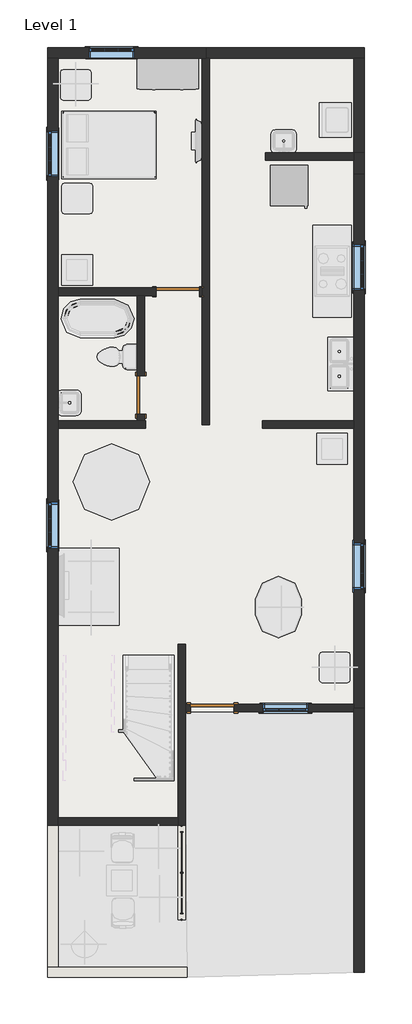
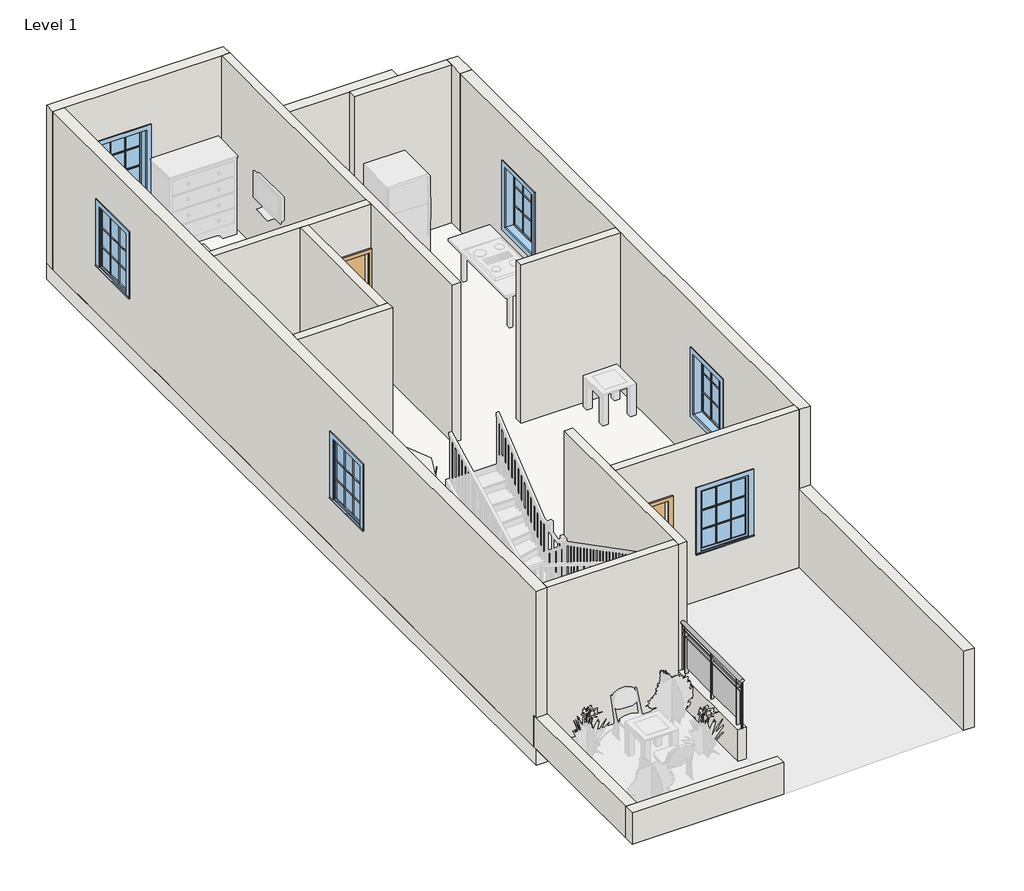
# One storey, part 1 of 3: 19 walls, 6 windows, 3 doors, 1 railing, 1 slab.
"""IFC4 building model written with IfcOpenShell, lengths in millimetres."""

from ifc_helpers import new_model, si_unit, point, frame, origin, origin_with_axes, place, context, project, spatial, polyline, ellipse_curve, trimmed, outline, extrude, faceted_brep, transform, mapped, element, save
from ifc_brep_helpers import plane_surface, extruded_surface, advanced_brep
from components import door_255cab33, door_b6e9fca3, door_99d96fc5, window_29c06734, window_5c190c7e

model = new_model("IFC4")

# Units and contexts
model_context = context("Model", 3, world=origin())
ifc_project = project(units=[si_unit("LENGTHUNIT", "METRE", prefix="MILLI")], contexts=[model_context])

# Site, building, storey
site = spatial("IfcSite", under=ifc_project)
building = spatial("IfcBuilding", under=site)
storey = spatial("IfcBuildingStorey", under=building, Name="Level 1", Elevation=0.0)

# Doors
placement = place(None, origin())
door_shape = door_255cab33(model_context)
element("IfcDoor", 1, ObjectType="Single-Flush : 30\" x 80\"", at=placement, inside=storey, context=model_context, shape_type="MappedRepresentation", body=[
    mapped(door_shape, transform((-1163.5479637, 6058.6104001, 0.0), x_axis=(0.0, -1.0, 0.0), y_axis=(1.0, 0.0, 0.0), z_axis=(0.0, 0.0, 1.0))),
])
door_2_shape = door_b6e9fca3(model_context)
element("IfcDoor", 2, ObjectType="Single-Flush : 34\" x 84\"", at=placement, inside=storey, context=model_context, shape_type="MappedRepresentation", body=[
    mapped(door_2_shape, transform((-426.9479637, 8116.0104001, 0.0), x_axis=(1.0, 0.0, 0.0), y_axis=(0.0, 1.0, 0.0), z_axis=(0.0, 0.0, 1.0))),
])
door_3_shape = door_99d96fc5(model_context)
element("IfcDoor", 3, ObjectType="Single-Flush : 34\" x 84\"", at=placement, inside=storey, context=model_context, shape_type="MappedRepresentation", body=[
    mapped(door_3_shape, transform((258.8520363, -164.3895999, 0.0), x_axis=(-1.0, 0.0, 0.0), y_axis=(0.0, -1.0, 0.0), z_axis=(0.0, 0.0, 1.0))),
])

# Railing
element("IfcRailing", 4, ObjectType="Glass Panel - Bottom Fill", at=placement, inside=storey, context=model_context, shape_type="SolidModel", body=[
    advanced_brep(
    [(-312.6479637, -2501.1895999, 1524.0), (-388.8479637, -2501.1895999, 1524.0), (-312.6479637, -4380.7895999, 1524.0), (-388.8479637, -4380.7895999, 1524.0)],
    [
        (0, 1, ellipse_curve(frame((-350.7479637, -2501.1895999, 1524.0), z_axis=(0.0, 1.0, 0.0), x_axis=(-1.0, 0.0, 0.0)), 38.1, 28.575)),
        (1, 0, ellipse_curve(frame((-350.7479637, -2501.1895999, 1524.0), z_axis=(0.0, 1.0, 0.0), x_axis=(-1.0, 0.0, 0.0)), 38.1, 28.575)),
        (2, 3, ellipse_curve(frame((-350.7479637, -4380.7895999, 1524.0), z_axis=(0.0, -1.0, 0.0), x_axis=(-1.0, 0.0, 0.0)), 38.1, 28.575)),
        (3, 2, ellipse_curve(frame((-350.7479637, -4380.7895999, 1524.0), z_axis=(0.0, -1.0, 0.0), x_axis=(-1.0, 0.0, 0.0)), 38.1, 28.575)),
        (0, 2),
        (3, 1),
    ],
    [
        plane_surface(frame((-350.7479637, -2501.1895999, 1524.0), z_axis=(0.0, 1.0, 0.0), x_axis=(0.0, 0.0, -1.0))),
        plane_surface(frame((-350.7479637, -4380.7895999, 1524.0), z_axis=(0.0, -1.0, 0.0), x_axis=(0.0, 0.0, -1.0))),
        extruded_surface(trimmed(ellipse_curve(frame((-350.7479637, -4380.7895999, 1524.0), z_axis=(0.0, 1.0, 0.0), x_axis=(-1.0, 0.0, 0.0)), 38.1, 28.575), [point((-312.6479637, -4380.7895999, 1524.0))], [point((-388.8479637, -4380.7895999, 1524.0))], True, "CARTESIAN"), (0.0, 1879.6000000000004, 0.0), 1879.6000000000004),
        extruded_surface(trimmed(ellipse_curve(frame((-350.7479637, -4380.7895999, 1524.0), z_axis=(0.0, 1.0, 0.0), x_axis=(-1.0, 0.0, 0.0)), 38.1, 28.575), [point((-388.8479637, -4380.7895999, 1524.0))], [point((-312.6479637, -4380.7895999, 1524.0))], True, "CARTESIAN"), (0.0, 1879.6000000000004, 0.0), 1879.6000000000004),
    ],
    [
        (0, [[1, 2]]),
        (1, [[3, 4]]),
        (2, [[-1, 5, -4, 6]]),
        (3, [[-2, -6, -3, -5]]),
    ],
),
    extrude(outline(polyline([(-363.4479637, -2501.1895999), (-338.0479637, -2501.1895999), (-338.0479637, -4380.7895999), (-363.4479637, -4380.7895999), (-363.4479637, -2501.1895999)])), frame((0.0, 0.0, 1409.7), z_axis=(0.0, 0.0, 1.0), x_axis=(1.0, 0.0, 0.0)), (0.0, 0.0, 1.0), 25.4),
    extrude(outline(polyline([(-363.4479637, -2501.1895999), (-338.0479637, -2501.1895999), (-338.0479637, -4380.7895999), (-363.4479637, -4380.7895999), (-363.4479637, -2501.1895999)])), frame((0.0, 0.0, 1308.1), z_axis=(0.0, 0.0, 1.0), x_axis=(1.0, 0.0, 0.0)), (0.0, 0.0, 1.0), 25.4),
    extrude(outline(polyline([(-376.1479637, -4247.4395999), (-325.3479637, -4247.4395999), (-325.3479637, -4260.1395999), (-376.1479637, -4260.1395999), (-376.1479637, -4247.4395999)])), frame((0.0, 0.0, 609.6), z_axis=(0.0, 0.0, 1.0), x_axis=(1.0, 0.0, 0.0)), (0.0, 0.0, 1.0), 885.6788223),
    extrude(outline(polyline([(-344.2128067, -3440.9895999), (-344.2128067, -4253.7895999), (-350.5628067, -4253.7895999), (-350.5628067, -3440.9895999), (-344.2128067, -3440.9895999)])), frame((0.0, 0.0, 711.2), z_axis=(0.0, 0.0, 1.0), x_axis=(1.0, 0.0, 0.0)), (0.0, 0.0, 1.0), 596.9),
    extrude(outline(polyline([(-376.1479637, -3434.6395999), (-325.3479637, -3434.6395999), (-325.3479637, -3447.3395999), (-376.1479637, -3447.3395999), (-376.1479637, -3434.6395999)])), frame((0.0, 0.0, 609.6), z_axis=(0.0, 0.0, 1.0), x_axis=(1.0, 0.0, 0.0)), (0.0, 0.0, 1.0), 885.6788223),
    extrude(outline(polyline([(-344.2128067, -2628.1895999), (-344.2128067, -3440.9895999), (-350.5628067, -3440.9895999), (-350.5628067, -2628.1895999), (-344.2128067, -2628.1895999)])), frame((0.0, 0.0, 711.2), z_axis=(0.0, 0.0, 1.0), x_axis=(1.0, 0.0, 0.0)), (0.0, 0.0, 1.0), 596.9),
    extrude(outline(polyline([(-376.1479637, -2621.8395999), (-325.3479637, -2621.8395999), (-325.3479637, -2634.5395999), (-376.1479637, -2634.5395999), (-376.1479637, -2621.8395999)])), frame((0.0, 0.0, 609.6), z_axis=(0.0, 0.0, 1.0), x_axis=(1.0, 0.0, 0.0)), (0.0, 0.0, 1.0), 885.6788223),
    extrude(outline(polyline([(-360.2729637, -4368.0895999), (-341.2229637, -4368.0895999), (-341.2229637, -4387.1395999), (-360.2729637, -4387.1395999), (-360.2729637, -4368.0895999)])), frame((0.0, 0.0, 609.6), z_axis=(0.0, 0.0, 1.0), x_axis=(1.0, 0.0, 0.0)), (0.0, 0.0, 1.0), 885.6788223),
    extrude(outline(polyline([(-360.2729637, -2494.8395999), (-341.2229637, -2494.8395999), (-341.2229637, -2513.8895999), (-360.2729637, -2513.8895999), (-360.2729637, -2494.8395999)])), frame((0.0, 0.0, 609.6), z_axis=(0.0, 0.0, 1.0), x_axis=(1.0, 0.0, 0.0)), (0.0, 0.0, 1.0), 885.6788223),
])

# Slab
element("IfcSlab", 5, ObjectType="Generic - 12\"", at=placement, inside=storey, context=model_context, shape_type="SweptSolid", body=[
    extrude(outline(polyline([(3281.4520363, 12967.4104001), (3281.4520363, -240.5895999), (-274.5479637, -240.5895999), (-274.5479637, -2501.1895999), (-3017.7479637, -2501.1895999), (-3017.7479637, 12967.4104001), (3281.4520363, 12967.4104001)])), frame((0.0, 0.0, -304.8), z_axis=(0.0, 0.0, 1.0), x_axis=(1.0, 0.0, 0.0)), (0.0, 0.0, 1.0), 304.8),
])

# Walls
element("IfcWall", 6, ObjectType="Generic - 2'", at=placement, inside=storey, context=model_context, shape_type="Brep", body=[
    faceted_brep([(-2814.5479637, -5320.5895999, 0.0), (-2814.5479637, -2501.1895999, 0.0), (-2814.5479637, -2424.9895999, 0.0), (-2814.5479637, -2424.9895999, 609.6), (-2814.5479637, -5320.5895999, 609.6), (-3017.7479637, -5320.5895999, 0.0), (-3017.7479637, -5320.5895999, 609.6), (-3017.7479637, -2424.9895999, 609.6), (-3017.7479637, -2424.9895999, 0.0)], [[[0, 1, 2, 3, 4]], [[5, 6, 7, 8]], [[2, 1, 0, 5, 8]], [[3, 2, 8, 7]], [[4, 3, 7, 6]], [[0, 4, 6, 5]]]),
])
element("IfcWall", 7, ObjectType="Generic - 2'", at=placement, inside=storey, context=model_context, shape_type="Brep", body=[
    faceted_brep([(3078.2520363, -164.3895999, 0.0), (3078.2520363, -240.5895999, 0.0), (3078.2520363, -5422.1895999, 0.0), (3078.2520363, -5422.1895999, 1524.0), (3078.2520363, -164.3895999, 1524.0), (3281.4520363, -164.3895999, 0.0), (3281.4520363, -164.3895999, 1524.0), (3281.4520363, -5422.1895999, 1524.0), (3281.4520363, -5422.1895999, 0.0)], [[[0, 1, 2, 3, 4]], [[5, 6, 7, 8]], [[2, 1, 0, 5, 8]], [[3, 2, 8, 7]], [[4, 3, 7, 6]], [[0, 4, 6, 5]]]),
])
element("IfcWall", 8, ObjectType="Generic - 2'", at=placement, inside=storey, context=model_context, shape_type="Brep", body=[
    faceted_brep([(-249.1479637, -5320.5895999, 0.0), (-2814.5479637, -5320.5895999, 0.0), (-3017.7479637, -5320.5895999, 0.0), (-3017.7479637, -5320.5895999, 609.6), (-2814.5479637, -5320.5895999, 609.6), (-249.1479637, -5320.5895999, 609.6), (-249.1479637, -5523.7895999, 0.0), (-249.1479637, -5523.7895999, 609.6), (-3017.7479637, -5523.7895999, 609.6), (-3017.7479637, -5523.7895999, 0.0)], [[[0, 1, 2, 3, 4, 5]], [[6, 7, 8, 9]], [[2, 1, 0, 6, 9]], [[5, 4, 3, 8, 7]], [[0, 5, 7, 6]], [[3, 2, 9, 8]]]),
])
element("IfcWall", 9, ObjectType="Generic - 6'", at=placement, inside=storey, context=model_context, shape_type="Brep", body=[
    faceted_brep([(55.6520363, 12764.2104001, 3048.0), (55.6520363, 12764.2104001, 0.0), (55.6520363, 8192.2104001, 0.0), (55.6520363, 8039.8104001, 0.0), (55.6520363, 5474.4104001, 0.0), (55.6520363, 5474.4104001, 3048.0), (55.6520363, 8039.8104001, 3048.0), (55.6520363, 8192.2104001, 3048.0), (208.0520363, 12764.2104001, 0.0), (208.0520363, 12764.2104001, 1524.0), (208.0520363, 12764.2104001, 3048.0), (208.0520363, 5474.4104001, 3048.0), (208.0520363, 5474.4104001, 0.0), (131.8520363, 12764.2104001, 0.0)], [[[0, 1, 2, 3, 4, 5, 6, 7]], [[8, 9, 10, 11, 12]], [[4, 3, 2, 1, 13, 8, 12]], [[5, 4, 12, 11]], [[0, 7, 6, 5, 11, 10]], [[0, 10, 9, 8, 13, 1]]]),
])
element("IfcWall", 10, ObjectType="Generic - 6'", at=placement, inside=storey, context=model_context, shape_type="SweptSolid", body=[
    extrude(outline(polyline([(1262.1520363, 5550.6104001), (3078.2520363, 5550.6104001), (3078.2520363, 5398.2104001), (1262.1520363, 5398.2104001), (1262.1520363, 5550.6104001)])), origin_with_axes(), (0.0, 0.0, 1.0), 3048.0),
])
element("IfcWall", 11, ObjectType="Generic - 6'", at=placement, inside=storey, context=model_context, shape_type="Brep", body=[
    faceted_brep([(4.8520363, 8039.8104001, 2133.6), (4.8520363, 8039.8104001, 0.0), (55.6520363, 8039.8104001, 0.0), (55.6520363, 8039.8104001, 3048.0), (-1087.3479637, 8039.8104001, 3048.0), (-1239.7479637, 8039.8104001, 3048.0), (-2814.5479637, 8039.8104001, 3048.0), (-2814.5479637, 8039.8104001, 0.0), (-1239.7479637, 8039.8104001, 0.0), (-1087.3479637, 8039.8104001, 0.0), (-858.7479637, 8039.8104001, 0.0), (-858.7479637, 8039.8104001, 2133.6), (55.6520363, 8192.2104001, 0.0), (4.8520363, 8192.2104001, 0.0), (4.8520363, 8192.2104001, 2133.6), (-858.7479637, 8192.2104001, 2133.6), (-858.7479637, 8192.2104001, 0.0), (-2814.5479637, 8192.2104001, 0.0), (-2814.5479637, 8192.2104001, 3048.0), (55.6520363, 8192.2104001, 3048.0)], [[[0, 1, 2, 3, 4, 5, 6, 7, 8, 9, 10, 11]], [[12, 13, 14, 15, 16, 17, 18, 19]], [[2, 1, 13, 12]], [[10, 9, 8, 7, 17, 16]], [[6, 5, 4, 3, 19, 18]], [[7, 6, 18, 17]], [[3, 2, 12, 19]], [[14, 13, 1, 0]], [[15, 14, 0, 11]], [[16, 15, 11, 10]]]),
])
element("IfcWall", 12, ObjectType="Generic - 6'", at=placement, inside=storey, context=model_context, shape_type="SweptSolid", body=[
    extrude(outline(polyline([(5677.6104001, 2032.0), (5677.6104001, 0.0), (5550.6104001, 0.0), (5550.6104001, 3048.0), (8039.8104001, 3048.0), (8039.8104001, 0.0), (6439.6104001, 0.0), (6439.6104001, 2032.0), (5677.6104001, 2032.0)])), frame((-1239.7479637, 0.0, 0.0), z_axis=(1.0, 0.0, 0.0), x_axis=(0.0, 1.0, 0.0)), (0.0, 0.0, 1.0), 152.4),
])
element("IfcWall", 13, ObjectType="Generic - 6'", at=placement, inside=storey, context=model_context, shape_type="Brep", body=[
    faceted_brep([(-172.9479637, -88.1895999, 2133.6), (-172.9479637, -88.1895999, 0.0), (-274.5479637, -88.1895999, 0.0), (-274.5479637, -88.1895999, 3048.0), (3078.2520363, -88.1895999, 3048.0), (3078.2520363, -88.1895999, 0.0), (690.6520363, -88.1895999, 0.0), (690.6520363, -88.1895999, 2133.6), (1262.1520363, -88.1895999, 2133.6), (1262.1520363, -88.1895999, 914.4), (2176.5520363, -88.1895999, 914.4), (2176.5520363, -88.1895999, 2133.6), (-274.5479637, -240.5895999, 0.0), (-172.9479637, -240.5895999, 0.0), (-172.9479637, -240.5895999, 2133.6), (690.6520363, -240.5895999, 2133.6), (690.6520363, -240.5895999, 0.0), (3078.2520363, -240.5895999, 0.0), (3078.2520363, -240.5895999, 1524.0), (3078.2520363, -240.5895999, 3048.0), (-274.5479637, -240.5895999, 3048.0), (1262.1520363, -240.5895999, 2133.6), (2176.5520363, -240.5895999, 2133.6), (2176.5520363, -240.5895999, 914.4), (1262.1520363, -240.5895999, 914.4), (3078.2520363, -164.3895999, 0.0)], [[[0, 1, 2, 3, 4, 5, 6, 7], [8, 9, 10, 11]], [[12, 13, 14, 15, 16, 17, 18, 19, 20], [21, 22, 23, 24]], [[6, 5, 25, 17, 16]], [[2, 1, 13, 12]], [[4, 3, 20, 19]], [[3, 2, 12, 20]], [[14, 13, 1, 0]], [[15, 14, 0, 7]], [[16, 15, 7, 6]], [[9, 8, 21, 24]], [[10, 9, 24, 23]], [[11, 10, 23, 22]], [[8, 11, 22, 21]], [[4, 19, 18, 17, 25, 5]]]),
])
element("IfcWall", 14, ObjectType="Generic - 6'", at=placement, inside=storey, context=model_context, shape_type="Brep", body=[
    faceted_brep([(-274.5479637, -4380.7895999, 0.0), (-274.5479637, -2424.9895999, 0.0), (-274.5479637, -2424.9895999, 609.6), (-274.5479637, -2501.1895999, 609.6), (-274.5479637, -4380.7895999, 609.6), (-426.9479637, -4380.7895999, 0.0), (-426.9479637, -4380.7895999, 609.6), (-426.9479637, -2501.1895999, 609.6), (-426.9479637, -2424.9895999, 609.6), (-426.9479637, -2424.9895999, 0.0), (-426.9479637, -2501.1895999, 0.0)], [[[0, 1, 2, 3, 4]], [[5, 6, 7, 8, 9, 10]], [[1, 0, 5, 10, 9]], [[2, 1, 9, 8]], [[4, 3, 2, 8, 7, 6]], [[0, 4, 6, 5]]]),
])
element("IfcWall", 15, ObjectType="Generic - 6'", at=placement, inside=storey, context=model_context, shape_type="Brep", body=[
    faceted_brep([(-2814.5479637, -2501.1895999, 3048.0), (-2814.5479637, -2501.1895999, 609.6), (-2814.5479637, -2501.1895999, 0.0), (-426.9479637, -2501.1895999, 0.0), (-426.9479637, -2501.1895999, 609.6), (-426.9479637, -2501.1895999, 3048.0), (-2814.5479637, -2348.7895999, 0.0), (-2814.5479637, -2348.7895999, 3048.0), (-426.9479637, -2348.7895999, 3048.0), (-426.9479637, -2348.7895999, 0.0), (-2814.5479637, -2424.9895999, 0.0), (-426.9479637, -2424.9895999, 0.0)], [[[0, 1, 2, 3, 4, 5]], [[6, 7, 8, 9]], [[3, 2, 10, 6, 9, 11]], [[0, 5, 8, 7]], [[0, 7, 6, 10, 2, 1]], [[3, 11, 9, 8, 5, 4]]]),
])
element("IfcWall", 16, ObjectType="Generic - 6'", at=placement, inside=storey, context=model_context, shape_type="Brep", body=[
    faceted_brep([(-1074.6479637, 5550.6104001, 0.0), (-1087.3479637, 5550.6104001, 0.0), (-1239.7479637, 5550.6104001, 0.0), (-2814.5479637, 5550.6104001, 0.0), (-2814.5479637, 5550.6104001, 3048.0), (-1239.7479637, 5550.6104001, 3048.0), (-1087.3479637, 5550.6104001, 3048.0), (-1074.6479637, 5550.6104001, 3048.0), (-1074.6479637, 5398.2104001, 0.0), (-1074.6479637, 5398.2104001, 3048.0), (-2814.5479637, 5398.2104001, 3048.0), (-2814.5479637, 5398.2104001, 0.0)], [[[0, 1, 2, 3, 4, 5, 6, 7]], [[8, 9, 10, 11]], [[3, 2, 1, 0, 8, 11]], [[7, 6, 5, 4, 10, 9]], [[0, 7, 9, 8]], [[4, 3, 11, 10]]]),
])
element("IfcWall", 17, ObjectType="Generic - 6'", at=placement, inside=storey, context=model_context, shape_type="SweptSolid", body=[
    extrude(outline(polyline([(3078.2520363, 10732.2104001), (1312.9520363, 10732.2104001), (1312.9520363, 10884.6104001), (3078.2520363, 10884.6104001), (3078.2520363, 10732.2104001)])), origin_with_axes(), (0.0, 0.0, 1.0), 3048.0),
])
element("IfcWall", 18, ObjectType="Generic - 6'", at=placement, inside=storey, context=model_context, shape_type="Brep", body=[
    faceted_brep([(-274.5479637, -2424.9895999, 0.0), (-274.5479637, -240.5895999, 0.0), (-274.5479637, -88.1895999, 0.0), (-274.5479637, 1105.6104001, 0.0), (-274.5479637, 1105.6104001, 3048.0), (-274.5479637, -88.1895999, 3048.0), (-274.5479637, -240.5895999, 3048.0), (-274.5479637, -2501.1895999, 3048.0), (-274.5479637, -2501.1895999, 609.6), (-274.5479637, -2424.9895999, 609.6), (-426.9479637, -2424.9895999, 0.0), (-426.9479637, -2424.9895999, 609.6), (-426.9479637, -2501.1895999, 609.6), (-426.9479637, -2501.1895999, 3048.0), (-426.9479637, -2348.7895999, 3048.0), (-426.9479637, 1105.6104001, 3048.0), (-426.9479637, 1105.6104001, 0.0), (-426.9479637, -2348.7895999, 0.0)], [[[0, 1, 2, 3, 4, 5, 6, 7, 8, 9]], [[10, 11, 12, 13, 14, 15, 16, 17]], [[3, 2, 1, 0, 10, 17, 16]], [[4, 3, 16, 15]], [[7, 6, 5, 4, 15, 14, 13]], [[0, 9, 11, 10]], [[8, 12, 11, 9]], [[8, 7, 13, 12]]]),
])
element("IfcWall", 19, ObjectType="Generic - 8\"", at=placement, inside=storey, context=model_context, shape_type="Brep", body=[
    faceted_brep([(-3017.7479637, 12764.2104001, 0.0), (-2814.5479637, 12764.2104001, 0.0), (55.6520363, 12764.2104001, 0.0), (131.8520363, 12764.2104001, 0.0), (131.8520363, 12764.2104001, 1524.0), (208.0520363, 12764.2104001, 1524.0), (208.0520363, 12764.2104001, 3048.0), (55.6520363, 12764.2104001, 3048.0), (-2814.5479637, 12764.2104001, 3048.0), (-3017.7479637, 12764.2104001, 3048.0), (-1290.5479637, 12764.2104001, 2133.6), (-1290.5479637, 12764.2104001, 914.4), (-2204.9479637, 12764.2104001, 914.4), (-2204.9479637, 12764.2104001, 2133.6), (-3017.7479637, 12967.4104001, 0.0), (-3017.7479637, 12967.4104001, 3048.0), (208.0520363, 12967.4104001, 3048.0), (208.0520363, 12967.4104001, 1524.0), (131.8520363, 12967.4104001, 1524.0), (131.8520363, 12967.4104001, 0.0), (-1290.5479637, 12967.4104001, 2133.6), (-2204.9479637, 12967.4104001, 2133.6), (-2204.9479637, 12967.4104001, 914.4), (-1290.5479637, 12967.4104001, 914.4)], [[[0, 1, 2, 3, 4, 5, 6, 7, 8, 9], [10, 11, 12, 13]], [[14, 15, 16, 17, 18, 19], [20, 21, 22, 23]], [[3, 2, 1, 0, 14, 19]], [[9, 8, 7, 6, 16, 15]], [[0, 9, 15, 14]], [[11, 10, 20, 23]], [[12, 11, 23, 22]], [[13, 12, 22, 21]], [[10, 13, 21, 20]], [[4, 3, 19, 18]], [[17, 5, 4, 18]], [[6, 5, 17, 16]]]),
])
element("IfcWall", 20, ObjectType="Generic - 8\"", at=placement, inside=storey, context=model_context, shape_type="SweptSolid", body=[
    extrude(outline(polyline([(3078.2520363, 10884.6104001), (3078.2520363, 12764.2104001), (3281.4520363, 12764.2104001), (3281.4520363, 10884.6104001), (3078.2520363, 10884.6104001)])), origin_with_axes(), (0.0, 0.0, 1.0), 1524.0),
])
element("IfcWall", 21, ObjectType="Generic - 8\"", at=placement, inside=storey, context=model_context, shape_type="Brep", body=[
    faceted_brep([(3078.2520363, 10884.6104001, 3048.0), (3078.2520363, 10884.6104001, 1524.0), (3078.2520363, 10884.6104001, 0.0), (3078.2520363, 10732.2104001, 0.0), (3078.2520363, 10452.8104001, 0.0), (3078.2520363, 10452.8104001, 3048.0), (3078.2520363, 10732.2104001, 3048.0), (3281.4520363, 10884.6104001, 0.0), (3281.4520363, 10884.6104001, 1524.0), (3281.4520363, 10884.6104001, 3048.0), (3281.4520363, 10452.8104001, 3048.0), (3281.4520363, 10452.8104001, 0.0)], [[[0, 1, 2, 3, 4, 5, 6]], [[7, 8, 9, 10, 11]], [[4, 3, 2, 7, 11]], [[5, 4, 11, 10]], [[0, 6, 5, 10, 9]], [[0, 9, 8, 7, 2, 1]]]),
])
element("IfcWall", 22, ObjectType="Generic - 8\"", at=placement, inside=storey, context=model_context, shape_type="Brep", body=[
    faceted_brep([(131.8520363, 12764.2104001, 0.0), (208.0520363, 12764.2104001, 0.0), (3078.2520363, 12764.2104001, 0.0), (3281.4520363, 12764.2104001, 0.0), (3281.4520363, 12764.2104001, 1524.0), (3078.2520363, 12764.2104001, 1524.0), (208.0520363, 12764.2104001, 1524.0), (131.8520363, 12764.2104001, 1524.0), (131.8520363, 12967.4104001, 0.0), (131.8520363, 12967.4104001, 1524.0), (208.0520363, 12967.4104001, 1524.0), (3281.4520363, 12967.4104001, 1524.0), (3281.4520363, 12967.4104001, 0.0)], [[[0, 1, 2, 3, 4, 5, 6, 7]], [[8, 9, 10, 11, 12]], [[3, 2, 1, 0, 8, 12]], [[7, 6, 5, 4, 11, 10, 9]], [[0, 7, 9, 8]], [[4, 3, 12, 11]]]),
])
element("IfcWall", 23, ObjectType="Generic - 8\"", at=placement, inside=storey, context=model_context, shape_type="Brep", body=[
    faceted_brep([(-2814.5479637, -2424.9895999, 0.0), (-2814.5479637, -2348.7895999, 0.0), (-2814.5479637, 5398.2104001, 0.0), (-2814.5479637, 5550.6104001, 0.0), (-2814.5479637, 8039.8104001, 0.0), (-2814.5479637, 8192.2104001, 0.0), (-2814.5479637, 12764.2104001, 0.0), (-2814.5479637, 12764.2104001, 3048.0), (-2814.5479637, 8192.2104001, 3048.0), (-2814.5479637, 8039.8104001, 3048.0), (-2814.5479637, 5550.6104001, 3048.0), (-2814.5479637, 5398.2104001, 3048.0), (-2814.5479637, -2348.7895999, 3048.0), (-2814.5479637, -2501.1895999, 3048.0), (-2814.5479637, -2501.1895999, 609.6), (-2814.5479637, -2424.9895999, 609.6), (-2814.5479637, 11316.4104001, 2133.6), (-2814.5479637, 11316.4104001, 914.4), (-2814.5479637, 10402.0104001, 914.4), (-2814.5479637, 10402.0104001, 2133.6), (-2814.5479637, 3925.0104001, 2133.6), (-2814.5479637, 3925.0104001, 914.4), (-2814.5479637, 3010.6104001, 914.4), (-2814.5479637, 3010.6104001, 2133.6), (-3017.7479637, -2424.9895999, 0.0), (-3017.7479637, -2424.9895999, 609.6), (-3017.7479637, -2501.1895999, 609.6), (-3017.7479637, -2501.1895999, 3048.0), (-3017.7479637, 12764.2104001, 3048.0), (-3017.7479637, 12764.2104001, 0.0), (-3017.7479637, 11316.4104001, 2133.6), (-3017.7479637, 10402.0104001, 2133.6), (-3017.7479637, 10402.0104001, 914.4), (-3017.7479637, 11316.4104001, 914.4), (-3017.7479637, 3925.0104001, 2133.6), (-3017.7479637, 3010.6104001, 2133.6), (-3017.7479637, 3010.6104001, 914.4), (-3017.7479637, 3925.0104001, 914.4)], [[[0, 1, 2, 3, 4, 5, 6, 7, 8, 9, 10, 11, 12, 13, 14, 15], [16, 17, 18, 19], [20, 21, 22, 23]], [[24, 25, 26, 27, 28, 29], [30, 31, 32, 33], [34, 35, 36, 37]], [[6, 5, 4, 3, 2, 1, 0, 24, 29]], [[13, 12, 11, 10, 9, 8, 7, 28, 27]], [[7, 6, 29, 28]], [[16, 19, 31, 30]], [[19, 18, 32, 31]], [[18, 17, 33, 32]], [[17, 16, 30, 33]], [[20, 23, 35, 34]], [[23, 22, 36, 35]], [[22, 21, 37, 36]], [[21, 20, 34, 37]], [[0, 15, 25, 24]], [[14, 26, 25, 15]], [[14, 13, 27, 26]]]),
])
element("IfcWall", 24, ObjectType="Generic - 8\"", at=placement, inside=storey, context=model_context, shape_type="Brep", body=[
    faceted_brep([(3078.2520363, 10452.8104001, 0.0), (3078.2520363, 5550.6104001, 0.0), (3078.2520363, 5398.2104001, 0.0), (3078.2520363, -88.1895999, 0.0), (3078.2520363, -164.3895999, 0.0), (3078.2520363, -164.3895999, 1524.0), (3078.2520363, -240.5895999, 1524.0), (3078.2520363, -240.5895999, 3048.0), (3078.2520363, -88.1895999, 3048.0), (3078.2520363, 5398.2104001, 3048.0), (3078.2520363, 5550.6104001, 3048.0), (3078.2520363, 10452.8104001, 3048.0), (3078.2520363, 2197.8104001, 2133.6), (3078.2520363, 2197.8104001, 914.4), (3078.2520363, 3112.2104001, 914.4), (3078.2520363, 3112.2104001, 2133.6), (3078.2520363, 8141.4104001, 2133.6), (3078.2520363, 8141.4104001, 914.4), (3078.2520363, 9055.8104001, 914.4), (3078.2520363, 9055.8104001, 2133.6), (3281.4520363, 10452.8104001, 0.0), (3281.4520363, 10452.8104001, 3048.0), (3281.4520363, -240.5895999, 3048.0), (3281.4520363, -240.5895999, 1524.0), (3281.4520363, -164.3895999, 1524.0), (3281.4520363, -164.3895999, 0.0), (3281.4520363, 2197.8104001, 2133.6), (3281.4520363, 3112.2104001, 2133.6), (3281.4520363, 3112.2104001, 914.4), (3281.4520363, 2197.8104001, 914.4), (3281.4520363, 8141.4104001, 2133.6), (3281.4520363, 9055.8104001, 2133.6), (3281.4520363, 9055.8104001, 914.4), (3281.4520363, 8141.4104001, 914.4)], [[[0, 1, 2, 3, 4, 5, 6, 7, 8, 9, 10, 11], [12, 13, 14, 15], [16, 17, 18, 19]], [[20, 21, 22, 23, 24, 25], [26, 27, 28, 29], [30, 31, 32, 33]], [[4, 3, 2, 1, 0, 20, 25]], [[11, 10, 9, 8, 7, 22, 21]], [[0, 11, 21, 20]], [[5, 4, 25, 24]], [[23, 6, 5, 24]], [[7, 6, 23, 22]], [[12, 15, 27, 26]], [[15, 14, 28, 27]], [[14, 13, 29, 28]], [[13, 12, 26, 29]], [[16, 19, 31, 30]], [[19, 18, 32, 31]], [[18, 17, 33, 32]], [[17, 16, 30, 33]]]),
])

# Windows
window_shape = window_29c06734(model_context)
element("IfcWindow", 25, ObjectType="Casement 3x3 with Trim : 36\" x 48\"", at=placement, inside=storey, context=model_context, shape_type="MappedRepresentation", body=[
    mapped(window_shape, transform((-1747.7479637, 12865.8104001, 0.0), x_axis=(1.0, 0.0, 0.0), y_axis=(0.0, 1.0, 0.0), z_axis=(0.0, 0.0, 1.0))),
])
element("IfcWindow", 26, ObjectType="Casement 3x3 with Trim : 36\" x 48\"", at=placement, inside=storey, context=model_context, shape_type="MappedRepresentation", body=[
    mapped(window_shape, transform((-2916.1479637, 10859.2104001, 0.0), x_axis=(0.0, 1.0, 0.0), y_axis=(-1.0, 0.0, 0.0), z_axis=(0.0, 0.0, 1.0))),
])
element("IfcWindow", 27, ObjectType="Casement 3x3 with Trim : 36\" x 48\"", at=placement, inside=storey, context=model_context, shape_type="MappedRepresentation", body=[
    mapped(window_shape, transform((-2916.1479637, 3467.8104001, 0.0), x_axis=(0.0, 1.0, 0.0), y_axis=(-1.0, 0.0, 0.0), z_axis=(0.0, 0.0, 1.0))),
])
element("IfcWindow", 28, ObjectType="Casement 3x3 with Trim : 36\" x 48\"", at=placement, inside=storey, context=model_context, shape_type="MappedRepresentation", body=[
    mapped(window_shape, transform((3179.8520363, 2655.0104001, 0.0), x_axis=(0.0, -1.0, 0.0), y_axis=(1.0, 0.0, 0.0), z_axis=(0.0, 0.0, 1.0))),
])
element("IfcWindow", 29, ObjectType="Casement 3x3 with Trim : 36\" x 48\"", at=placement, inside=storey, context=model_context, shape_type="MappedRepresentation", body=[
    mapped(window_shape, transform((3179.8520363, 8598.6104001, 0.0), x_axis=(0.0, -1.0, 0.0), y_axis=(1.0, 0.0, 0.0), z_axis=(0.0, 0.0, 1.0))),
])
window_2_shape = window_5c190c7e(model_context)
element("IfcWindow", 30, ObjectType="Casement 3x3 with Trim : 36\" x 48\"", at=placement, inside=storey, context=model_context, shape_type="MappedRepresentation", body=[
    mapped(window_2_shape, transform((1719.3520363, -164.3895999, 0.0), x_axis=(-1.0, 0.0, 0.0), y_axis=(0.0, -1.0, 0.0), z_axis=(0.0, 0.0, 1.0))),
])

save(model, "model.ifc")

# Revit data of these elements
# Type "Single-Flush : 30\" x 80\""
#   Type Mark = "5"
#   Construction Type Id = "MDOOR"
#   Assembly Code = "C1020"
#   Analytic Construction = "Metal"
#   Thickness = 0' - 2"
#   Heat Transfer Coefficient (U) = 0.651978 BTU/(h·ft²·°F)
#   Height = 6' - 8"
#   Trim Projection Ext = 0' - 1"
#   Trim Projection Int = 0' - 1"
#   Trim Width = 0' - 3"
#   Width = 2' - 6"
#   Define Thermal Properties by = 1
#   Door Material = Door - Panel
#   Frame Material = Door - Frame
#   Visual Light Transmittance = 0
#   Solar Heat Gain Coefficient = 0
#   Function = (empty or 0)
#   Wall Closure = (empty or 0)
# Type "Single-Flush : 34\" x 84\""
#   Type Mark = "2"
#   Construction Type Id = "MDOOR"
#   Assembly Code = "C1020"
#   Analytic Construction = "Metal"
#   Thickness = 0' - 2"
#   Heat Transfer Coefficient (U) = 0.651978 BTU/(h·ft²·°F)
#   Height = 7' - 0"
#   Trim Projection Ext = 0' - 1"
#   Trim Projection Int = 0' - 1"
#   Trim Width = 0' - 3"
#   Width = 2' - 10"
#   Define Thermal Properties by = 1
#   Door Material = Door - Panel
#   Frame Material = Door - Frame
#   Visual Light Transmittance = 0
#   Solar Heat Gain Coefficient = 0
#   Function = (empty or 0)
#   Wall Closure = (empty or 0)
# Type "Glass Panel - Bottom Fill"
#   Assembly Code = "C2010400"
#   built-in parameter 1008612 = 0.0416667 (stored number, unit not read)
#   built-in parameter 1008611 = 0.0416667 (stored number, unit not read)
#   built-in parameter 1008609 = 0.333333 (stored number, unit not read)
#   built-in parameter 1008604 = 0.166667 (stored number, unit not read)
#   built-in parameter 1008603 = 0.166667 (stored number, unit not read)
#   Railing Height = 3' - 0"
#   built-in parameter 1008630 = 2
#   built-in parameter 1008610 = 2
#   built-in parameter 1008618 = Baluster - Square : 3/4"
# Type "Generic - 12\""
#   Assembly Code = "B1010"
#   Function = 0
#   Layers, outside or top first: 1' - 0" no material (function 1)
# Type "Generic - 2'"
#   Assembly Code = "B2010"
#   Layers, outside or top first: 0' - 8" "Birch" (function 1)
# Type "Generic - 6'"
#   Assembly Code = "B2010"
#   Layers, outside or top first: 0' - 6" "Brick, Common" (function 1)
# Type "Generic - 8\""
#   Assembly Code = "B2010"
#   Layers, outside or top first: 0' - 8" "Brick, Common" (function 1)
# Type "Casement 3x3 with Trim : 36\" x 48\""
#   Type Mark = "10"
#   Construction Type Id = "GSP4R"
#   Assembly Code = "B2020100"
#   Analytic Construction = "1/8 in Pilkington single glazing"
#   Visual Light Transmittance = 0.9
#   Solar Heat Gain Coefficient = 0.78
#   Heat Transfer Coefficient (U) = 0.6496 BTU/(h·ft²·°F)
#   Height = 4' - 0"
#   Default Sill Height = 3' - 0"
#   Trim Projection - Ext. = 0' - 0 1/2"
#   Trim Projection - Int. = 0' - 0 3/4"
#   Trim Width - Exterior = 0' - 3 1/2"
#   Trim Width - Interior = 0' - 3 1/2"
#   Width = 3' - 0"
#   Window Inset = 0' - 0 3/4"
#   Define Thermal Properties by = 1
#   Glass Pane Material = Glass
#   Sash Material = Sash
#   Trim Exterior Material = Trim
#   Trim Interior Material = Trim
#   Wall Closure = (empty or 0)
# Element 1 (IfcDoor, "Single-Flush : 30\" x 80\"")
#   Phase Created = New Construction
#   Materials on its faces: "Door - Frame", "Door - Panel"
# Elements 2, 3 (IfcDoor, "Single-Flush : 34\" x 84\"")
#   Phase Created = New Construction
#   Materials on its faces: "Door - Frame", "Door - Panel"
# Element 4 (IfcRailing, "Glass Panel - Bottom Fill")
#   built-in parameter 1008621 = 2 (stored number, unit not read)
#   Phase Created = New Construction
#   Materials on its faces: "Glass"
# Element 5 (IfcSlab, "Generic - 12\"")
#   Height Offset From Level = 0' - 0"
#   Phase Created = New Construction
#   Materials on its faces: "Default Floor"
# Elements 6, 8 (IfcWall, "Generic - 2'")
#   Top Offset = 0' - 0"
#   Base Offset = 0' - 0"
#   Unconnected Height = 2' - 0"
#   wall height = 2' - 0"
#   Phase Created = New Construction
#   Base Constraint = Level 1
#   Materials on its faces: "Birch"
# Element 7 (IfcWall, "Generic - 2'")
#   Top Offset = 0' - 0"
#   Base Offset = 0' - 0"
#   Unconnected Height = 5' - 0"
#   wall height = 5' - 0"
#   Phase Created = New Construction
#   Base Constraint = Level 1
#   Materials on its faces: "Birch"
# Elements 9, 10, 11, 12, 13, 15, 16, 17, 18 (IfcWall, "Generic - 6'")
#   Top Offset = 0' - 0"
#   Base Offset = 0' - 0"
#   Unconnected Height = 10' - 0"
#   wall height = 10' - 0"
#   Phase Created = New Construction
#   Base Constraint = Level 1
#   Materials on its faces: "Brick, Common"
# Element 14 (IfcWall, "Generic - 6'")
#   Top Offset = 0' - 0"
#   Base Offset = 0' - 0"
#   Unconnected Height = 2' - 0"
#   wall height = 2' - 0"
#   Phase Created = New Construction
#   Base Constraint = Level 1
#   Materials on its faces: "Brick, Common"
# Elements 19, 21, 23, 24 (IfcWall, "Generic - 8\"")
#   Top Offset = 0' - 0"
#   Base Offset = 0' - 0"
#   Unconnected Height = 10' - 0"
#   wall height = 10' - 0"
#   Phase Created = New Construction
#   Base Constraint = Level 1
#   Materials on its faces: "Brick, Common"
# Elements 20, 22 (IfcWall, "Generic - 8\"")
#   Top Offset = 0' - 0"
#   Base Offset = 0' - 0"
#   Unconnected Height = 5' - 0"
#   wall height = 5' - 0"
#   Phase Created = New Construction
#   Base Constraint = Level 1
#   Materials on its faces: "Brick, Common"
# Element 25 (IfcWindow, "Casement 3x3 with Trim : 36\" x 48\"")
#   Mark = "1"
#   Phase Created = New Construction
#   Materials on its faces: "Sash", "Glass", "Trim"
# Element 26 (IfcWindow, "Casement 3x3 with Trim : 36\" x 48\"")
#   Mark = "2"
#   Phase Created = New Construction
#   Materials on its faces: "Sash", "Glass", "Trim"
# Element 27 (IfcWindow, "Casement 3x3 with Trim : 36\" x 48\"")
#   Mark = "3"
#   Phase Created = New Construction
#   Materials on its faces: "Sash", "Glass", "Trim"
# Element 28 (IfcWindow, "Casement 3x3 with Trim : 36\" x 48\"")
#   Mark = "5"
#   Phase Created = New Construction
#   Materials on its faces: "Sash", "Glass", "Trim"
# Element 29 (IfcWindow, "Casement 3x3 with Trim : 36\" x 48\"")
#   Mark = "6"
#   Phase Created = New Construction
#   Materials on its faces: "Sash", "Glass", "Trim"
# Element 30 (IfcWindow, "Casement 3x3 with Trim : 36\" x 48\"")
#   Mark = "4"
#   Phase Created = New Construction
#   Materials on its faces: "Sash", "Glass", "Trim"
# Materials
#   "Door - Panel": class "Wood", colour RGB 210 159 95, transparency 0
#   "Door - Frame": colour RGB 118 70 51, transparency 0
#   "Birch": class "Wood", colour RGB 224 178 126, transparency 0, Description = "Betula Alleghaniensis", Cost = 0
#   "Brick, Common": class "Masonry", colour RGB 170 98 104, transparency 0, Description = "Common brick", Cost = 0
#   "Glass": class "Glass", colour RGB 0 128 192, transparency 0.75, Description = "Soda Lime Glass", Cost = 0
#   "Sash": class "Wood", colour RGB 224 178 126, transparency 0
#   "Trim": class "Wood", colour RGB 224 178 126, transparency 0
#   "Default Floor": colour RGB 128 128 128, transparency 0
# Room at (-1445.696, 10652.182) mm, phase "New Construction", upper level "Level 1", upper offset 10' - 0", lower offset 0' - 0"
#   Number = "1"
#   Name = "BEDROOM"
# Room at (-2085.795, 6783.872) mm, phase "New Construction", upper level "Level 1", upper offset 10' - 0", lower offset 0' - 0"
#   Number = "2"
#   Name = "TOILET"
# Room at (1683.82, 11714.335) mm, phase "New Construction", upper level "Level 1", upper offset 10' - 0", lower offset 0' - 0"
#   Number = "3"
# Room at (1425.012, 8046.028) mm, phase "New Construction", upper level "Level 1", upper offset 10' - 0", lower offset 0' - 0"
#   Number = "4"
#   Name = "KITCHEN"
# Room at (427.298, 3110.475) mm, phase "New Construction", upper level "Level 1", upper offset 10' - 0", lower offset 0' - 0"
#   Number = "5"
